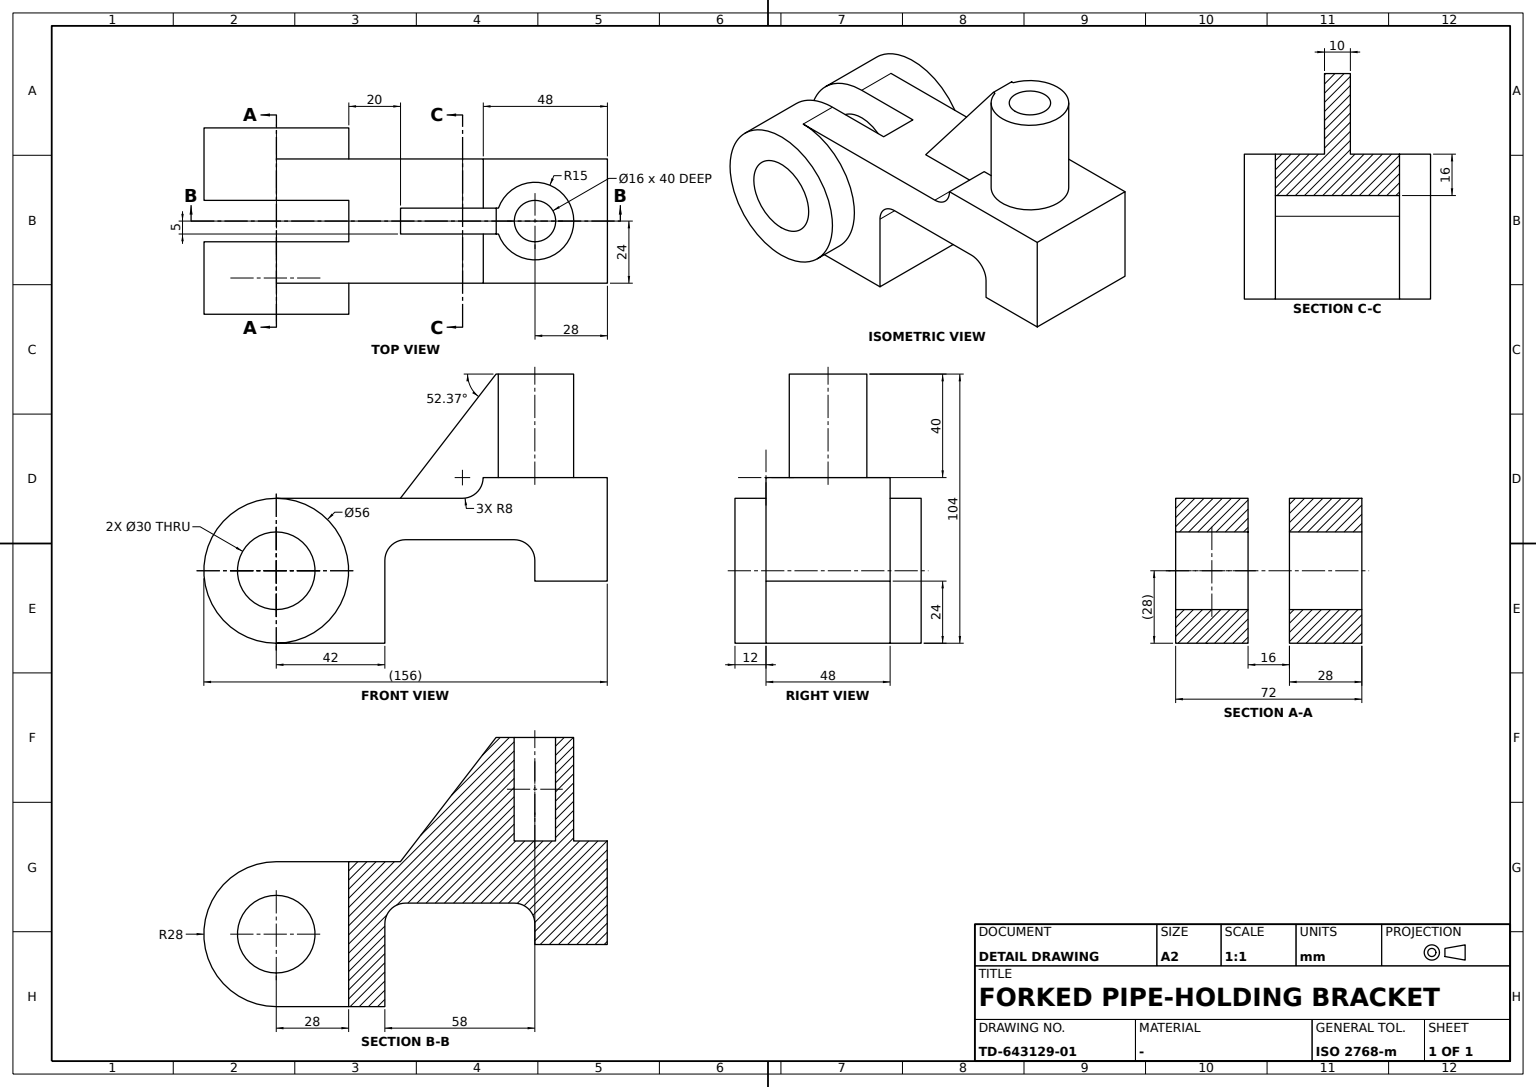
CATIA V5 part; units mm, degrees
sketch "Sketch1" plane through (0, 0, 0) normal (1, 0, 0) x (0, 1, 0)
  arc A0 (0, -28) -> (0, 28) centre (0, 0) ccw
  line L0 (0, 28) -> (72, 28)
  point P0 (0, 28)
  point P1 (80, 28.0216)
  point P2 (80, 36)
  line L1 (80, 36) -> (128, 36)
  line L2 (128, 36) -> (128, -4)
  line L3 (128, -4) -> (100, -4)
  point P3 (100, -4)
  line L4 (92, 12) -> (50, 12)
  point P4 (42.5878, 4)
  line L5 (42, 4) -> (42, -28)
  line L6 (42, -28) -> (0, -28)
  arc A1 (50, 12) -> (42, 4) centre (50, 4) ccw
  arc A2 (80, 36) -> (72, 28) centre (72, 36) cw
  point P5 (80, 36)
  point P6 (72, 36)
  line L7 (100, -4) -> (100, 4)
  arc A3 (92, 12) -> (100, 4) centre (92, 4) cw
  dimension "radius A0" = 28
  dimension "length L1" = 48
  dimension "length L2" = 40
  dimension "length L3" = 28
  dimension "radius A1" = 8
  dimension "radius A2" = 8
  dimension "distance L4 L0" = 16
  dimension "distance L1 L0" = 8
  dimension "distance y axis P6" = 72
  dimension "distance P3 L5" = 58
  dimension "radius A3" = 8
  constraint coincidence P0 y-axis
  constraint coincidence P5 P2
  constraint tangency L0 A0
  constraint tangency L6 A0
  constraint tangency A1 L4
  constraint tangency A1 L5
  constraint tangency A2 L0
  constraint tangency A3 L4
  constraint tangency A3 L7
  constraint horizontal L1 x-axis
  constraint horizontal L3 x-axis
  constraint horizontal L4 x-axis
  constraint horizontal L6 x-axis
  constraint horizontal L0 x-axis
  constraint vertical L2 y-axis
  constraint vertical L5 y-axis
  constraint vertical L7 y-axis
extrude "Pad1" add sketch "Sketch1" along normal mid plane 48
sketch "Sketch2" plane through (0, 0, 28) normal (0, 0, 1) x (1, 0, 0)
  line L0 (-8, 28) -> (8, 28)
  line L1 (8, 28) -> (8, 0)
  line L2 (8, 0) -> (-8, 0)
  line L3 (-8, 0) -> (-8, 28)
  line L4 (-24, 0) -> (24, 0) construction
  dimension "length L1" = 28
  dimension "length L2" = 16
  dimension "distance L1 y axis" = 8
  constraint horizontal L0 x-axis
  constraint horizontal L2 x-axis
  constraint vertical L1 y-axis
  constraint vertical L3 y-axis
  constraint coincidence L2 L4
extrude "Pocket1" cut sketch "Sketch2" against normal blind 72
sketch "Sketch3" plane through (-8, 0, 0) normal (1, 0, 0) x (0, 1, 0)
  circle A0 centre (0, 0) radius 28
  arc A1 (0, -28) -> (0, 28) centre (0, 0) ccw construction
  arc A2 (0, -28) -> (0, 28) centre (0, 0) ccw construction
  circle A3 centre (0, 0) radius 15
  dimension "radius A3" = 15
  constraint concentricity A0 A1
  constraint coincidence A0 A2
extrude "Pad2" add sketch "Sketch3" against normal blind 28
mirror "Mirror1" about plane through (0, 0, 0) normal (1, 0, 0) of "Pad2"
sketch "Sketch4" plane through (0, 0, 36) normal (0, 0, 1) x (1, 0, 0)
  circle A0 centre (0, 100) radius 15
  point P0 (0, 100)
  circle A1 centre (0, 100) radius 8
  line L0 (-24, 80) -> (24, 80) construction
  dimension "radius A0" = 15
  dimension "radius A1" = 8
  dimension "distance P0 L0" = 20
  constraint coincidence P0 y-axis
extrude "Pad3" add sketch "Sketch4" along normal blind 40
sketch "Sketch5" plane through (0, 0, 0) normal (1, 0, 0) x (0, 1, 0)
  line L0 (48, 28) -> (72, 28)
  point P0 (48, 28)
  point P1 (72, 28)
  line L1 (72, 28) -> (0, 28) construction
  point P2 (28, 28)
  arc A0 (72, 28) -> (80, 36) centre (72, 36) ccw
  point P3 (72, 28)
  line L2 (80, 36) -> (85, 36)
  point P4 (85, 36)
  line L3 (85, 36) -> (85, 76)
  point P5 (85, 36)
  line L4 (80, 36) -> (128, 36) construction
  line L5 (85, 76) -> (48, 28)
  point P6 (48, 28)
  dimension "distance P2 P0" = 20
  dimension "length L3" = 40
  dimension "D3" = 15
  constraint horizontal L0 x-axis
  constraint horizontal L2 x-axis
  constraint coincidence L0 L1
  constraint coincidence P1 P3
  constraint coincidence P5 L4
  constraint coincidence P4 P5
  constraint coincidence L5 P0
  constraint coincidence P0 P6
  constraint vertical L3 y-axis
extrude "Pad4" add sketch "Sketch5" along normal mid plane 10
sketch "Sketch6" plane through (0, 85, 0) normal (0, 1, 0) x (-1, 0, 0)
  line L0 (5, 76) -> (-5, 76)
  line L1 (-5, 36) -> (-5, 76)
  line L2 (5, 36) -> (-5, 36)
  line L3 (5, 36) -> (5, 76)
extrude "Pad5" add sketch "Sketch6" along normal blind 5
equation "\"radius A1@Sketch1\" = deleted_LENGTH"
